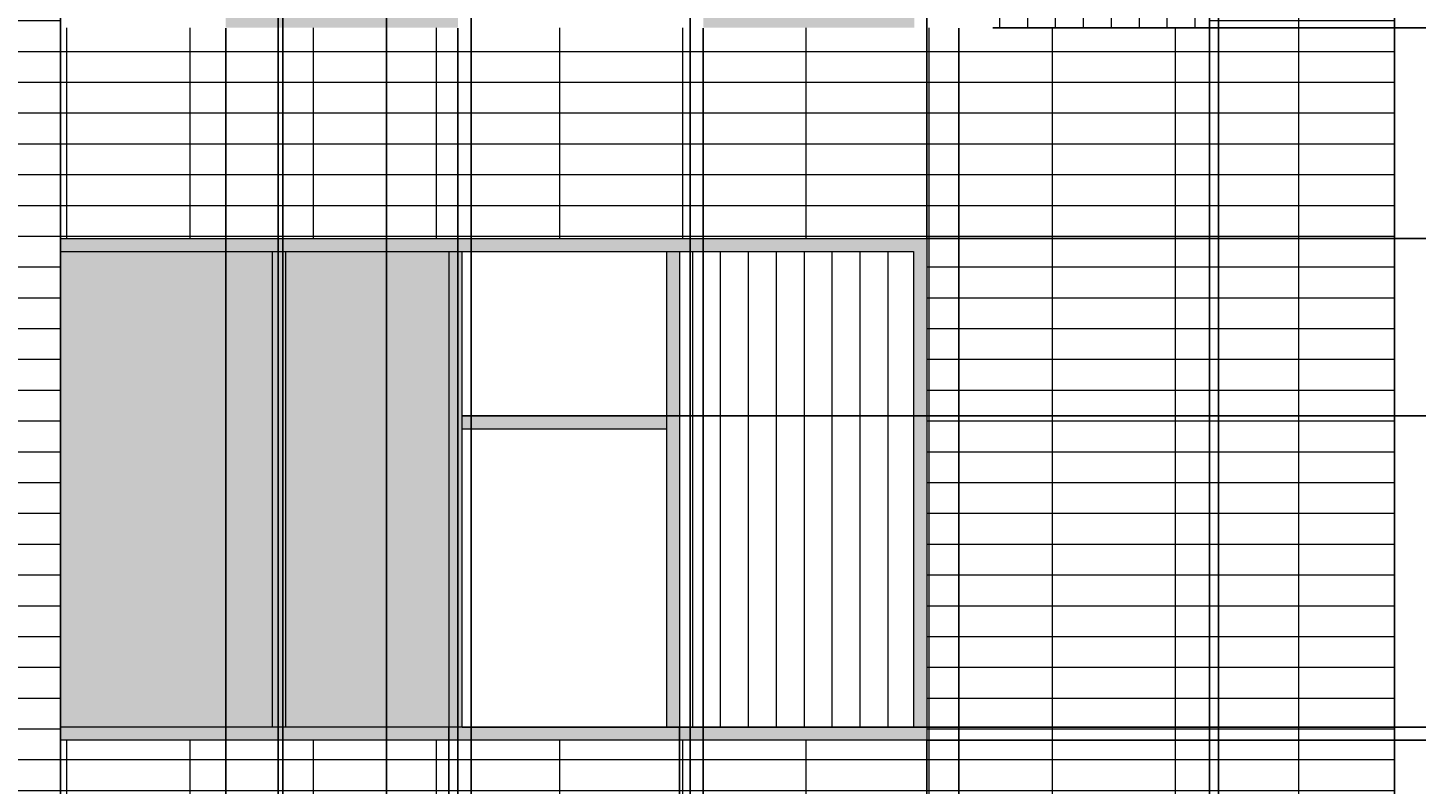
# Model space of a CAD drawing. Units: inches. Extents: x 241 to 943, y 109 to 1396.
# Tile 15 of 34: x 613 to 824, y 620 to 735. Entities that reach past the tile are written whole.
import ezdxf

# ---------------------------------------------------------------- set-up
doc = ezdxf.new("R2010")
doc.units = ezdxf.units.IN
doc.header["$MEASUREMENT"] = 0
for name, color, linetype, lineweight in [('A-ANNO-DIMS', 2, 'Continuous', 18), ('A-ELEV', 7, 'Continuous', 25), ('A-ELEV-SHAD', 9, 'Continuous', 13), ('A-GLAZ', 4, 'Continuous', 18), ('A-GLAZ-PATT', 18, 'Continuous', 13), ('A-WALL-PATT', 8, 'Continuous', 13)]:
    doc.layers.add(name, color=color, linetype=linetype, lineweight=lineweight)
doc.styles.get("Standard").update_dxf_attribs({"font": 'arial.ttf'})
doc.dimstyles.get("Standard").update_dxf_attribs({"dimtxt": 1.4375, "dimasz": 0.18, "dimexe": 0.18, "dimexo": 0.0625, "dimgap": 0.09, "dimtad": 0, "dimtih": 1, "dimtoh": 1, "dimdec": 4, "dimzin": 0, "dimdsep": 46, "dimlunit": 4, "dimtxsty": 'Standard', "dimcen": 0.09, "dimadec": 0, "dimazin": 0, "dimtfac": 1, "dimtdec": 4, "dimtofl": 0, "dimtmove": 0, "dimatfit": 3, "dimfxl": 1, "dimtolj": 1, "dimtzin": 0, "dimarcsym": 0})

# ---------------------------------------------------------------- blocks, each defined once
blk = doc.blocks.new('*D6')
at = {"layer": 'A-ANNO-DIMS', "color": 0, "lineweight": -2, "transparency": 16777216}
for p, q in [((820.84, 232.89), (820.84, 1395.05)), ((881.67, 232.89), (881.67, 1395.05)), ((821.02, 1394.87), (848.73, 1394.87)), ((881.49, 1394.87), (853.77, 1394.87))]:
    blk.add_line(p, q, dxfattribs=at)
at = {"layer": 'A-ANNO-DIMS', "color": 0, "transparency": 16777216}
for points in [[(821.02, 1394.9), (821.02, 1394.84), (820.84, 1394.87)], [(881.49, 1394.9), (881.49, 1394.84), (881.67, 1394.87)]]:
    blk.add_solid(points, dxfattribs=at)
at = {"layer": 'Defpoints', "color": 0, "transparency": 16777216}
for p in [(881.67, 1394.87), (820.84, 232.83), (881.67, 232.83)]:
    blk.add_point(p, dxfattribs=at)
at = {"layer": 'A-ANNO-DIMS', "color": 0, "transparency": 16777216, "insert": (851.25, 1394.87), "char_height": 1.438, "attachment_point": 5}
blk.add_mtext('\\A1;60.83', dxfattribs=at)
blk = doc.blocks.new('*D12')
at = {"layer": 'A-ANNO-DIMS', "color": 0, "lineweight": -2, "transparency": 16777216}
for p, q in [((530.23, 384.24), (530.23, 1395.05)), ((650.91, 384.24), (650.91, 1395.05)), ((530.41, 1394.87), (587.56, 1394.87)), ((650.73, 1394.87), (593.58, 1394.87))]:
    blk.add_line(p, q, dxfattribs=at)
at = {"layer": 'A-ANNO-DIMS', "color": 0, "transparency": 16777216}
for points in [[(530.41, 1394.9), (530.41, 1394.84), (530.23, 1394.87)], [(650.73, 1394.9), (650.73, 1394.84), (650.91, 1394.87)]]:
    blk.add_solid(points, dxfattribs=at)
at = {"layer": 'Defpoints', "color": 0, "transparency": 16777216}
for p in [(650.91, 1394.87), (530.23, 384.18), (650.91, 384.18)]:
    blk.add_point(p, dxfattribs=at)
at = {"layer": 'A-ANNO-DIMS', "color": 0, "transparency": 16777216, "insert": (590.57, 1394.87), "char_height": 1.438, "attachment_point": 5}
blk.add_mtext('\\A1;120.68', dxfattribs=at)
blk = doc.blocks.new('*D13')
at = {"layer": 'A-ANNO-DIMS', "color": 0, "lineweight": -2, "transparency": 16777216}
for p, q in [((650.91, 384.24), (650.91, 1395.05)), ((667.39, 290.06), (667.39, 1395.05)), ((651.09, 1394.87), (656.14, 1394.87)), ((667.21, 1394.87), (662.16, 1394.87))]:
    blk.add_line(p, q, dxfattribs=at)
at = {"layer": 'A-ANNO-DIMS', "color": 0, "transparency": 16777216}
for points in [[(651.09, 1394.9), (651.09, 1394.84), (650.91, 1394.87)], [(667.21, 1394.9), (667.21, 1394.84), (667.39, 1394.87)]]:
    blk.add_solid(points, dxfattribs=at)
at = {"layer": 'Defpoints', "color": 0, "transparency": 16777216}
for p in [(667.39, 1394.87), (650.91, 384.18), (667.39, 290)]:
    blk.add_point(p, dxfattribs=at)
at = {"layer": 'A-ANNO-DIMS', "color": 0, "transparency": 16777216, "insert": (659.15, 1394.87), "char_height": 1.438, "attachment_point": 5}
blk.add_mtext('\\A1;16.486', dxfattribs=at)
blk = doc.blocks.new('*D14')
at = {"layer": 'A-ANNO-DIMS', "color": 0, "lineweight": -2, "transparency": 16777216}
for p, q in [((667.39, 290.06), (667.39, 1395.05)), ((794.03, 290.06), (794.03, 1395.05)), ((667.57, 1394.87), (727.7, 1394.87)), ((793.85, 1394.87), (733.72, 1394.87))]:
    blk.add_line(p, q, dxfattribs=at)
at = {"layer": 'A-ANNO-DIMS', "color": 0, "transparency": 16777216}
for points in [[(667.57, 1394.9), (667.57, 1394.84), (667.39, 1394.87)], [(793.85, 1394.9), (793.85, 1394.84), (794.03, 1394.87)]]:
    blk.add_solid(points, dxfattribs=at)
at = {"layer": 'Defpoints', "color": 0, "transparency": 16777216}
for p in [(794.03, 1394.87), (667.39, 290), (794.03, 290)]:
    blk.add_point(p, dxfattribs=at)
at = {"layer": 'A-ANNO-DIMS', "color": 0, "transparency": 16777216, "insert": (730.71, 1394.87), "char_height": 1.438, "attachment_point": 5}
blk.add_mtext('\\A1;126.63', dxfattribs=at)
blk = doc.blocks.new('*D15')
at = {"layer": 'A-ANNO-DIMS', "color": 0, "lineweight": -2, "transparency": 16777216}
for p, q in [((794.03, 290.06), (794.03, 1395.05)), ((820.84, 232.89), (820.84, 1395.05)), ((794.21, 1394.87), (805.04, 1394.87)), ((820.66, 1394.87), (809.82, 1394.87))]:
    blk.add_line(p, q, dxfattribs=at)
at = {"layer": 'A-ANNO-DIMS', "color": 0, "transparency": 16777216}
for points in [[(794.21, 1394.9), (794.21, 1394.84), (794.03, 1394.87)], [(820.66, 1394.9), (820.66, 1394.84), (820.84, 1394.87)]]:
    blk.add_solid(points, dxfattribs=at)
at = {"layer": 'Defpoints', "color": 0, "transparency": 16777216}
for p in [(820.84, 1394.87), (794.03, 290), (820.84, 232.83)]:
    blk.add_point(p, dxfattribs=at)
at = {"layer": 'A-ANNO-DIMS', "color": 0, "transparency": 16777216, "insert": (807.43, 1394.87), "char_height": 1.438, "attachment_point": 5}
blk.add_mtext('\\A1;26.81', dxfattribs=at)
blk = doc.blocks.new('*D46')
at = {"layer": 'A-ANNO-DIMS', "color": 0, "lineweight": -2, "transparency": 16777216}
for p, q in [((749.7, 702.79), (940.6, 702.79)), ((940.42, 702.61), (940.42, 665.42)), ((940.42, 626.58), (940.42, 663.77)), ((749.7, 626.4), (940.6, 626.4))]:
    blk.add_line(p, q, dxfattribs=at)
at = {"layer": 'A-ANNO-DIMS', "color": 0, "transparency": 16777216}
for points in [[(940.39, 702.61), (940.45, 702.61), (940.42, 702.79)], [(940.39, 626.58), (940.45, 626.58), (940.42, 626.4)]]:
    blk.add_solid(points, dxfattribs=at)
at = {"layer": 'Defpoints', "color": 0, "transparency": 16777216}
for p in [(749.63, 702.79), (940.42, 702.79), (749.63, 626.4)]:
    blk.add_point(p, dxfattribs=at)
at = {"layer": 'A-ANNO-DIMS', "color": 0, "transparency": 16777216, "insert": (940.42, 664.6), "char_height": 1.438, "attachment_point": 5}
blk.add_mtext('\\A1;76.39', dxfattribs=at)
blk = doc.blocks.new('*D47')
at = {"layer": 'A-ANNO-DIMS', "color": 0, "lineweight": -2, "transparency": 16777216}
for p, q in [((792.75, 841.54), (940.6, 841.54)), ((940.42, 841.36), (940.42, 789.02)), ((940.42, 735.03), (940.42, 787.37)), ((792.75, 734.85), (940.6, 734.85))]:
    blk.add_line(p, q, dxfattribs=at)
at = {"layer": 'A-ANNO-DIMS', "color": 0, "transparency": 16777216}
for points in [[(940.39, 841.36), (940.45, 841.36), (940.42, 841.54)], [(940.39, 735.03), (940.45, 735.03), (940.42, 734.85)]]:
    blk.add_solid(points, dxfattribs=at)
at = {"layer": 'Defpoints', "color": 0, "transparency": 16777216}
for p in [(792.69, 841.54), (940.42, 841.54), (792.69, 734.85)]:
    blk.add_point(p, dxfattribs=at)
at = {"layer": 'A-ANNO-DIMS', "color": 0, "transparency": 16777216, "insert": (940.42, 788.2), "char_height": 1.438, "attachment_point": 5}
blk.add_mtext('\\A1;106.68', dxfattribs=at)
blk = doc.blocks.new('*D63')
at = {"layer": 'A-ANNO-DIMS', "color": 0, "lineweight": -2, "transparency": 16777216}
for p, q in [((651.6, 568.89), (651.6, 1395.05)), ((792.69, 568.89), (792.69, 1395.05)), ((651.78, 1394.87), (719.84, 1394.87)), ((792.51, 1394.87), (724.45, 1394.87))]:
    blk.add_line(p, q, dxfattribs=at)
at = {"layer": 'A-ANNO-DIMS', "color": 0, "transparency": 16777216}
for points in [[(651.78, 1394.9), (651.78, 1394.84), (651.6, 1394.87)], [(792.51, 1394.9), (792.51, 1394.84), (792.69, 1394.87)]]:
    blk.add_solid(points, dxfattribs=at)
at = {"layer": 'Defpoints', "color": 0, "transparency": 16777216}
for p in [(792.69, 1394.87), (651.6, 568.83), (792.69, 568.83)]:
    blk.add_point(p, dxfattribs=at)
at = {"layer": 'A-ANNO-DIMS', "color": 0, "transparency": 16777216, "insert": (722.14, 1394.87), "char_height": 1.438, "attachment_point": 5}
blk.add_mtext('\\A1;141.1', dxfattribs=at)
blk = doc.blocks.new('*D64')
at = {"layer": 'A-ANNO-DIMS', "color": 0, "lineweight": -2, "transparency": 16777216}
for p, q in [((792.69, 568.89), (792.69, 1395.05)), ((820.84, 568.89), (820.84, 1395.05)), ((792.87, 1394.87), (803.68, 1394.87)), ((820.66, 1394.87), (809.85, 1394.87))]:
    blk.add_line(p, q, dxfattribs=at)
at = {"layer": 'A-ANNO-DIMS', "color": 0, "transparency": 16777216}
for points in [[(792.87, 1394.9), (792.87, 1394.84), (792.69, 1394.87)], [(820.66, 1394.9), (820.66, 1394.84), (820.84, 1394.87)]]:
    blk.add_solid(points, dxfattribs=at)
at = {"layer": 'Defpoints', "color": 0, "transparency": 16777216}
for p in [(820.84, 1394.87), (792.69, 568.83), (820.84, 568.83)]:
    blk.add_point(p, dxfattribs=at)
at = {"layer": 'A-ANNO-DIMS', "color": 0, "transparency": 16777216, "insert": (806.76, 1394.87), "char_height": 1.438, "attachment_point": 5}
blk.add_mtext('\\A1;28.146', dxfattribs=at)
blk = doc.blocks.new('*D66')
at = {"layer": 'A-ANNO-DIMS', "color": 0, "lineweight": -2, "transparency": 16777216}
for p, q in [((617.76, 702.85), (617.76, 1395.05)), ((749.63, 702.85), (749.63, 1395.05)), ((617.94, 1394.87), (680.69, 1394.87)), ((749.45, 1394.87), (686.7, 1394.87))]:
    blk.add_line(p, q, dxfattribs=at)
at = {"layer": 'A-ANNO-DIMS', "color": 0, "transparency": 16777216}
for points in [[(617.94, 1394.9), (617.94, 1394.84), (617.76, 1394.87)], [(749.45, 1394.9), (749.45, 1394.84), (749.63, 1394.87)]]:
    blk.add_solid(points, dxfattribs=at)
at = {"layer": 'Defpoints', "color": 0, "transparency": 16777216}
for p in [(749.63, 1394.87), (617.76, 702.79), (749.63, 702.79)]:
    blk.add_point(p, dxfattribs=at)
at = {"layer": 'A-ANNO-DIMS', "color": 0, "transparency": 16777216, "insert": (683.7, 1394.87), "char_height": 1.438, "attachment_point": 5}
blk.add_mtext('\\A1;131.87', dxfattribs=at)
blk = doc.blocks.new('*D82')
at = {"layer": 'A-ANNO-DIMS', "color": 0, "lineweight": -2, "transparency": 16777216}
for p, q in [((565.2, 568.89), (565.2, 1395.05)), ((651.6, 568.89), (651.6, 1395.05)), ((565.38, 1394.87), (605.89, 1394.87)), ((651.42, 1394.87), (610.91, 1394.87))]:
    blk.add_line(p, q, dxfattribs=at)
at = {"layer": 'A-ANNO-DIMS', "color": 0, "transparency": 16777216}
for points in [[(565.38, 1394.9), (565.38, 1394.84), (565.2, 1394.87)], [(651.42, 1394.9), (651.42, 1394.84), (651.6, 1394.87)]]:
    blk.add_solid(points, dxfattribs=at)
at = {"layer": 'Defpoints', "color": 0, "transparency": 16777216}
for p in [(651.6, 1394.87), (565.2, 568.83), (651.6, 568.83)]:
    blk.add_point(p, dxfattribs=at)
at = {"layer": 'A-ANNO-DIMS', "color": 0, "transparency": 16777216, "insert": (608.4, 1394.87), "char_height": 1.438, "attachment_point": 5}
blk.add_mtext('\\A1;86.40', dxfattribs=at)
blk = doc.blocks.new('*D83')
at = {"layer": 'A-ANNO-DIMS', "color": 0, "lineweight": -2, "transparency": 16777216}
for p, q in [((592.95, 700.85), (592.95, 1395.05)), ((617.76, 702.85), (617.76, 1395.05)), ((593.13, 1394.87), (602.27, 1394.87)), ((617.58, 1394.87), (608.45, 1394.87))]:
    blk.add_line(p, q, dxfattribs=at)
at = {"layer": 'A-ANNO-DIMS', "color": 0, "transparency": 16777216}
for points in [[(593.13, 1394.9), (593.13, 1394.84), (592.95, 1394.87)], [(617.58, 1394.9), (617.58, 1394.84), (617.76, 1394.87)]]:
    blk.add_solid(points, dxfattribs=at)
at = {"layer": 'Defpoints', "color": 0, "transparency": 16777216}
for p in [(617.76, 1394.87), (617.76, 702.79), (592.95, 700.79)]:
    blk.add_point(p, dxfattribs=at)
at = {"layer": 'A-ANNO-DIMS', "color": 0, "transparency": 16777216, "insert": (605.36, 1394.87), "char_height": 1.438, "attachment_point": 5}
blk.add_mtext('\\A1;24.805', dxfattribs=at)
blk = doc.blocks.new('*D84')
at = {"layer": 'A-ANNO-DIMS', "color": 0, "lineweight": -2, "transparency": 16777216}
for p, q in [((749.63, 702.85), (749.63, 1395.05)), ((820.84, 736.89), (820.84, 1395.05)), ((749.81, 1394.87), (782.73, 1394.87)), ((820.66, 1394.87), (787.74, 1394.87))]:
    blk.add_line(p, q, dxfattribs=at)
at = {"layer": 'A-ANNO-DIMS', "color": 0, "transparency": 16777216}
for points in [[(749.81, 1394.9), (749.81, 1394.84), (749.63, 1394.87)], [(820.66, 1394.9), (820.66, 1394.84), (820.84, 1394.87)]]:
    blk.add_solid(points, dxfattribs=at)
at = {"layer": 'Defpoints', "color": 0, "transparency": 16777216}
for p in [(820.84, 1394.87), (820.84, 736.83), (749.63, 702.79)]:
    blk.add_point(p, dxfattribs=at)
at = {"layer": 'A-ANNO-DIMS', "color": 0, "transparency": 16777216, "insert": (785.24, 1394.87), "char_height": 1.438, "attachment_point": 5}
blk.add_mtext('\\A1;71.20', dxfattribs=at)
blk = doc.blocks.new('*D85')
at = {"layer": 'A-ANNO-DIMS', "color": 0, "lineweight": -2, "transparency": 16777216}
for p, q in [((749.7, 626.4), (940.6, 626.4)), ((940.42, 626.22), (940.42, 598.44)), ((940.42, 569.01), (940.42, 596.79)), ((792.75, 568.83), (940.6, 568.83))]:
    blk.add_line(p, q, dxfattribs=at)
at = {"layer": 'A-ANNO-DIMS', "color": 0, "transparency": 16777216}
for points in [[(940.39, 626.22), (940.45, 626.22), (940.42, 626.4)], [(940.39, 569.01), (940.45, 569.01), (940.42, 568.83)]]:
    blk.add_solid(points, dxfattribs=at)
at = {"layer": 'Defpoints', "color": 0, "transparency": 16777216}
for p in [(749.63, 626.4), (940.42, 626.4), (792.69, 568.83)]:
    blk.add_point(p, dxfattribs=at)
at = {"layer": 'A-ANNO-DIMS', "color": 0, "transparency": 16777216, "insert": (940.42, 597.62), "char_height": 1.438, "attachment_point": 5}
blk.add_mtext('\\A1;57.57', dxfattribs=at)
blk = doc.blocks.new('*D86')
at = {"layer": 'A-ANNO-DIMS', "color": 0, "lineweight": -2, "transparency": 16777216}
for p, q in [((792.75, 734.85), (940.6, 734.85)), ((940.42, 734.67), (940.42, 719.65)), ((940.42, 702.97), (940.42, 718)), ((749.7, 702.79), (940.6, 702.79))]:
    blk.add_line(p, q, dxfattribs=at)
at = {"layer": 'A-ANNO-DIMS', "color": 0, "transparency": 16777216}
for points in [[(940.39, 734.67), (940.45, 734.67), (940.42, 734.85)], [(940.39, 702.97), (940.45, 702.97), (940.42, 702.79)]]:
    blk.add_solid(points, dxfattribs=at)
at = {"layer": 'Defpoints', "color": 0, "transparency": 16777216}
for p in [(792.69, 734.85), (940.42, 734.85), (749.63, 702.79)]:
    blk.add_point(p, dxfattribs=at)
at = {"layer": 'A-ANNO-DIMS', "color": 0, "transparency": 16777216, "insert": (940.42, 718.82), "char_height": 1.438, "attachment_point": 5}
blk.add_mtext('\\A1;32.06', dxfattribs=at)
blk = doc.blocks.new('*D99')
at = {"layer": 'A-ANNO-DIMS', "color": 0, "lineweight": -2, "transparency": 16777216}
for p, q in [((417.09, 181.71), (417.09, 1395.05)), ((667.39, 214.58), (667.39, 1395.05)), ((417.27, 1394.87), (539.16, 1394.87)), ((667.21, 1394.87), (545.33, 1394.87))]:
    blk.add_line(p, q, dxfattribs=at)
at = {"layer": 'A-ANNO-DIMS', "color": 0, "transparency": 16777216}
for points in [[(417.27, 1394.9), (417.27, 1394.84), (417.09, 1394.87)], [(667.21, 1394.9), (667.21, 1394.84), (667.39, 1394.87)]]:
    blk.add_solid(points, dxfattribs=at)
at = {"layer": 'Defpoints', "color": 0, "transparency": 16777216}
for p in [(667.39, 1394.87), (667.39, 214.52), (417.09, 181.65)]:
    blk.add_point(p, dxfattribs=at)
at = {"layer": 'A-ANNO-DIMS', "color": 0, "transparency": 16777216, "insert": (542.24, 1394.87), "char_height": 1.438, "attachment_point": 5}
blk.add_mtext('\\A1;250.30', dxfattribs=at)
blk = doc.blocks.new('*D119')
at = {"layer": 'A-ANNO-DIMS', "color": 0, "lineweight": -2, "transparency": 16777216}
for p, q in [((617.76, 734.79), (617.76, 109.81)), ((642.92, 734.79), (642.92, 109.81)), ((617.94, 109.99), (627.81, 109.99)), ((642.74, 109.99), (632.87, 109.99))]:
    blk.add_line(p, q, dxfattribs=at)
at = {"layer": 'A-ANNO-DIMS', "color": 0, "transparency": 16777216}
for points in [[(617.94, 110.02), (617.94, 109.96), (617.76, 109.99)], [(642.74, 110.02), (642.74, 109.96), (642.92, 109.99)]]:
    blk.add_solid(points, dxfattribs=at)
at = {"layer": 'Defpoints', "color": 0, "transparency": 16777216}
for p in [(617.76, 734.85), (642.92, 734.85), (642.92, 109.99)]:
    blk.add_point(p, dxfattribs=at)
at = {"layer": 'A-ANNO-DIMS', "color": 0, "transparency": 16777216, "insert": (630.34, 109.99), "char_height": 1.438, "attachment_point": 5}
blk.add_mtext('\\A1;25.16', dxfattribs=at)
blk = doc.blocks.new('*D120')
at = {"layer": 'A-ANNO-DIMS', "color": 0, "lineweight": -2, "transparency": 16777216}
for p, q in [((642.92, 734.79), (642.92, 109.81)), ((678.27, 734.79), (678.27, 109.81)), ((643.1, 109.99), (658.07, 109.99)), ((678.09, 109.99), (663.11, 109.99))]:
    blk.add_line(p, q, dxfattribs=at)
at = {"layer": 'A-ANNO-DIMS', "color": 0, "transparency": 16777216}
for points in [[(643.1, 110.02), (643.1, 109.96), (642.92, 109.99)], [(678.09, 110.02), (678.09, 109.96), (678.27, 109.99)]]:
    blk.add_solid(points, dxfattribs=at)
at = {"layer": 'Defpoints', "color": 0, "transparency": 16777216}
for p in [(642.92, 734.85), (678.27, 734.85), (678.27, 109.99)]:
    blk.add_point(p, dxfattribs=at)
at = {"layer": 'A-ANNO-DIMS', "color": 0, "transparency": 16777216, "insert": (660.59, 109.99), "char_height": 1.438, "attachment_point": 5}
blk.add_mtext('\\A1;35.35', dxfattribs=at)
blk = doc.blocks.new('*D121')
at = {"layer": 'A-ANNO-DIMS', "color": 0, "lineweight": -2, "transparency": 16777216}
for p, q in [((680.27, 736.86), (680.27, 109.81)), ((713.62, 736.86), (713.62, 109.81)), ((680.45, 109.99), (693.87, 109.99)), ((713.44, 109.99), (700.02, 109.99))]:
    blk.add_line(p, q, dxfattribs=at)
at = {"layer": 'A-ANNO-DIMS', "color": 0, "transparency": 16777216}
for points in [[(680.45, 110.02), (680.45, 109.96), (680.27, 109.99)], [(713.44, 110.02), (713.44, 109.96), (713.62, 109.99)]]:
    blk.add_solid(points, dxfattribs=at)
at = {"layer": 'Defpoints', "color": 0, "transparency": 16777216}
for p in [(680.27, 736.92), (713.62, 736.92), (713.62, 109.99)]:
    blk.add_point(p, dxfattribs=at)
at = {"layer": 'A-ANNO-DIMS', "color": 0, "transparency": 16777216, "insert": (696.95, 109.99), "char_height": 1.438, "attachment_point": 5}
blk.add_mtext('\\A1;33.356', dxfattribs=at)
blk = doc.blocks.new('*D122')
at = {"layer": 'A-ANNO-DIMS', "color": 0, "lineweight": -2, "transparency": 16777216}
for p, q in [((715.62, 734.79), (715.62, 109.81)), ((754.54, 734.79), (754.54, 109.81)), ((715.8, 109.99), (732.7, 109.99)), ((754.36, 109.99), (737.46, 109.99))]:
    blk.add_line(p, q, dxfattribs=at)
at = {"layer": 'A-ANNO-DIMS', "color": 0, "transparency": 16777216}
for points in [[(715.8, 110.02), (715.8, 109.96), (715.62, 109.99)], [(754.36, 110.02), (754.36, 109.96), (754.54, 109.99)]]:
    blk.add_solid(points, dxfattribs=at)
at = {"layer": 'Defpoints', "color": 0, "transparency": 16777216}
for p in [(715.62, 734.85), (754.54, 734.85), (754.54, 109.99)]:
    blk.add_point(p, dxfattribs=at)
at = {"layer": 'A-ANNO-DIMS', "color": 0, "transparency": 16777216, "insert": (735.08, 109.99), "char_height": 1.438, "attachment_point": 5}
blk.add_mtext('\\A1;38.91', dxfattribs=at)
blk = doc.blocks.new('*D123')
at = {"layer": 'A-ANNO-DIMS', "color": 0, "lineweight": -2, "transparency": 16777216}
for p, q in [((754.54, 734.79), (754.54, 109.81)), ((792.69, 734.79), (792.69, 109.81)), ((754.72, 109.99), (771.09, 109.99)), ((792.51, 109.99), (776.13, 109.99))]:
    blk.add_line(p, q, dxfattribs=at)
at = {"layer": 'A-ANNO-DIMS', "color": 0, "transparency": 16777216}
for points in [[(754.72, 110.02), (754.72, 109.96), (754.54, 109.99)], [(792.51, 110.02), (792.51, 109.96), (792.69, 109.99)]]:
    blk.add_solid(points, dxfattribs=at)
at = {"layer": 'Defpoints', "color": 0, "transparency": 16777216}
for p in [(754.54, 734.85), (792.69, 734.85), (792.69, 109.99)]:
    blk.add_point(p, dxfattribs=at)
at = {"layer": 'A-ANNO-DIMS', "color": 0, "transparency": 16777216, "insert": (773.61, 109.99), "char_height": 1.438, "attachment_point": 5}
blk.add_mtext('\\A1;38.15', dxfattribs=at)
blk = doc.blocks.new('*D125')
at = {"layer": 'A-ANNO-DIMS', "color": 0, "lineweight": -2, "transparency": 16777216}
for p, q in [((754.6, 799.98), (940.6, 799.98)), ((940.42, 799.8), (940.42, 768.24)), ((940.42, 735.03), (940.42, 766.59)), ((759.69, 734.85), (940.6, 734.85))]:
    blk.add_line(p, q, dxfattribs=at)
at = {"layer": 'A-ANNO-DIMS', "color": 0, "transparency": 16777216}
for points in [[(940.39, 799.8), (940.45, 799.8), (940.42, 799.98)], [(940.39, 735.03), (940.45, 735.03), (940.42, 734.85)]]:
    blk.add_solid(points, dxfattribs=at)
at = {"layer": 'Defpoints', "color": 0, "transparency": 16777216}
for p in [(754.54, 799.98), (940.42, 799.98), (759.62, 734.85)]:
    blk.add_point(p, dxfattribs=at)
at = {"layer": 'A-ANNO-DIMS', "color": 0, "transparency": 16777216, "insert": (940.42, 767.42), "char_height": 1.438, "attachment_point": 5}
blk.add_mtext('\\A1;65.13', dxfattribs=at)
blk = doc.blocks.new('*D132')
at = {"layer": 'A-ANNO-DIMS', "color": 0, "lineweight": -2, "transparency": 16777216}
for p, q in [((676.87, 628.34), (676.87, 109.81)), ((617.76, 626.34), (617.76, 109.81)), ((617.94, 109.99), (644.94, 109.99)), ((676.69, 109.99), (649.69, 109.99))]:
    blk.add_line(p, q, dxfattribs=at)
at = {"layer": 'A-ANNO-DIMS', "color": 0, "transparency": 16777216}
for points in [[(617.94, 110.02), (617.94, 109.96), (617.76, 109.99)], [(676.69, 110.02), (676.69, 109.96), (676.87, 109.99)]]:
    blk.add_solid(points, dxfattribs=at)
at = {"layer": 'Defpoints', "color": 0, "transparency": 16777216}
for p in [(676.87, 628.4), (617.76, 626.4), (676.87, 109.99)]:
    blk.add_point(p, dxfattribs=at)
at = {"layer": 'A-ANNO-DIMS', "color": 0, "transparency": 16777216, "insert": (647.31, 109.99), "char_height": 1.438, "attachment_point": 5}
blk.add_mtext('\\A1;59.11', dxfattribs=at)
blk = doc.blocks.new('*D133')
at = {"layer": 'A-ANNO-DIMS', "color": 0, "lineweight": -2, "transparency": 16777216}
for p, q in [((676.87, 628.34), (676.87, 109.81)), ((712.02, 628.34), (712.02, 109.81)), ((677.05, 109.99), (691.92, 109.99)), ((711.84, 109.99), (696.96, 109.99))]:
    blk.add_line(p, q, dxfattribs=at)
at = {"layer": 'A-ANNO-DIMS', "color": 0, "transparency": 16777216}
for points in [[(677.05, 110.02), (677.05, 109.96), (676.87, 109.99)], [(711.84, 110.02), (711.84, 109.96), (712.02, 109.99)]]:
    blk.add_solid(points, dxfattribs=at)
at = {"layer": 'Defpoints', "color": 0, "transparency": 16777216}
for p in [(676.87, 628.4), (712.02, 628.4), (712.02, 109.99)]:
    blk.add_point(p, dxfattribs=at)
at = {"layer": 'A-ANNO-DIMS', "color": 0, "transparency": 16777216, "insert": (694.44, 109.99), "char_height": 1.438, "attachment_point": 5}
blk.add_mtext('\\A1;35.15', dxfattribs=at)
blk = doc.blocks.new('*D134')
at = {"layer": 'A-ANNO-DIMS', "color": 0, "lineweight": -2, "transparency": 16777216}
for p, q in [((712.02, 628.34), (712.02, 109.81)), ((749.63, 626.34), (749.63, 109.81)), ((712.2, 109.99), (727.75, 109.99)), ((749.45, 109.99), (733.9, 109.99))]:
    blk.add_line(p, q, dxfattribs=at)
at = {"layer": 'A-ANNO-DIMS', "color": 0, "transparency": 16777216}
for points in [[(712.2, 110.02), (712.2, 109.96), (712.02, 109.99)], [(749.45, 110.02), (749.45, 109.96), (749.63, 109.99)]]:
    blk.add_solid(points, dxfattribs=at)
at = {"layer": 'Defpoints', "color": 0, "transparency": 16777216}
for p in [(712.02, 628.4), (749.63, 626.4), (749.63, 109.99)]:
    blk.add_point(p, dxfattribs=at)
at = {"layer": 'A-ANNO-DIMS', "color": 0, "transparency": 16777216, "insert": (730.82, 109.99), "char_height": 1.438, "attachment_point": 5}
blk.add_mtext('\\A1;37.616', dxfattribs=at)
blk = doc.blocks.new('*D135')
at = {"layer": 'A-ANNO-DIMS', "color": 0, "lineweight": -2, "transparency": 16777216}
for p, q in [((678.93, 675.79), (940.6, 675.79)), ((940.42, 675.61), (940.42, 652.92)), ((940.42, 628.58), (940.42, 651.27)), ((678.93, 628.4), (940.6, 628.4))]:
    blk.add_line(p, q, dxfattribs=at)
at = {"layer": 'A-ANNO-DIMS', "color": 0, "transparency": 16777216}
for points in [[(940.39, 675.61), (940.45, 675.61), (940.42, 675.79)], [(940.39, 628.58), (940.45, 628.58), (940.42, 628.4)]]:
    blk.add_solid(points, dxfattribs=at)
at = {"layer": 'Defpoints', "color": 0, "transparency": 16777216}
for p in [(678.87, 675.79), (940.42, 675.79), (678.87, 628.4)]:
    blk.add_point(p, dxfattribs=at)
at = {"layer": 'A-ANNO-DIMS', "color": 0, "transparency": 16777216, "insert": (940.42, 652.09), "char_height": 1.438, "attachment_point": 5}
blk.add_mtext('\\A1;47.38', dxfattribs=at)

msp = doc.modelspace()

# ---------------------------------------------------------------- hatches: boundary and pattern name
at = {"layer": 'A-ELEV-SHAD'}
h = msp.add_hatch(color=256, dxfattribs=at)
h.dxf.hatch_style = 1
h.paths.add_polyline_path([(537.4269, 566.8295), (534.1778, 566.8295), (534.1778, 527.3816), (537.4269, 527.3816)])
h.paths.add_polyline_path([(508.0803, 566.8295), (450.9259, 566.8295), (450.9259, 527.3816), (452.9259, 527.3816), (452.9259, 564.8295), (506.0803, 564.8295), (506.0803, 527.3816), (508.0803, 527.3816)])
h.paths.add_polyline_path([(481.5031, 564.8295), (479.5031, 564.8295), (479.5031, 527.3816), (481.5031, 527.3816)], flags=17)
h.paths.add_polyline_path([(481.5031, 525.3816), (479.5031, 525.3816), (479.5031, 521.3754), (481.5031, 521.3754)], flags=17)
h.paths.add_polyline_path([(508.0803, 525.3816), (506.0803, 525.3816), (506.0803, 521.3754), (452.9259, 521.3754), (452.9259, 525.3816), (450.9259, 525.3816), (450.9259, 519.3754), (508.0803, 519.3754)])
h.paths.add_polyline_path([(537.4269, 525.3816), (534.1778, 525.3816), (534.1778, 508.9074), (537.4269, 508.9074)])
h.paths.add_polyline_path([(749.6328, 702.7912), (617.7594, 702.7912), (617.7594, 700.7912), (747.6328, 700.7912), (747.6328, 628.4013), (617.7594, 628.4013), (617.7594, 626.4013), (749.6328, 626.4013)])
h.paths.add_polyline_path([(652.0129, 700.7912), (650.0129, 700.7912), (650.0129, 628.4013), (652.0129, 628.4013)], flags=17)
h.paths.add_polyline_path([(678.8698, 700.7912), (676.8698, 700.7912), (676.8698, 628.4013), (678.8698, 628.4013)], flags=17)
h.paths.add_polyline_path([(712.0171, 700.7912), (710.0171, 700.7912), (710.0171, 628.4013), (712.0171, 628.4013)], flags=17)
h.paths.add_polyline_path([(710.0171, 675.7856), (678.8698, 675.7856), (678.8698, 673.7856), (710.0171, 673.7856)], flags=17)
h.paths.add_polyline_path([(537.4269, 698.7912), (534.1778, 698.7912), (534.1778, 659.3434), (537.4269, 659.3434)], flags=0)
h.paths.add_polyline_path([(592.9542, 700.7912), (424.1086, 700.7912), (424.1086, 628.4013), (592.9542, 628.4013)])
h.paths.add_polyline_path([(590.8792, 698.7912), (590.8792, 630.4013), (426.1086, 630.4013), (426.1086, 698.7912)], flags=16)
h.paths.add_polyline_path([(563.2023, 698.7912), (563.2023, 659.3434), (563.9297, 659.3434), (563.9297, 651.3371), (508.1906, 651.3371), (508.0803, 651.3371), (450.9259, 651.3371), (428.0291, 651.3371), (428.0291, 698.7912), (451.9767, 698.7912), (508.0803, 698.7912), (537.4269, 698.7912)], flags=0)
h.paths.add_polyline_path([(506.0803, 696.7912), (506.0803, 653.3371), (452.9259, 653.3371), (452.9259, 657.3434), (445.5808, 657.3434, -1), (445.5808, 659.3434), (452.9259, 659.3434), (452.9259, 696.7912)], flags=0)
h.paths.add_polyline_path([(563.9297, 698.7912), (563.2023, 698.7912), (563.2023, 659.3434), (563.9297, 659.3434)], flags=0)
at = {"layer": 'A-GLAZ-PATT'}
h = msp.add_hatch(dxfattribs=at)
h.set_pattern_fill('GOST_GLASS', color=256, scale=0.89)
h.set_pattern_definition([(45, (0, 0), (7.5519, 0), [4.45, -6.23]), (45, (1.888, 0), (7.5519, 0), [1.78, -8.9]), (45, (0, 1.888), (7.5519, 0), [1.78, -8.9])])
h.paths.add_polyline_path([(676.8698, 700.7912), (652.0129, 700.7912), (652.0129, 628.4013), (676.8698, 628.4013)])
h.paths.add_polyline_path([(650.0129, 700.7912), (617.7594, 700.7912), (617.7594, 628.4013), (650.0129, 628.4013)])
h.paths.add_polyline_path([(747.7579, 841.5382), (715.6236, 841.5382), (715.6236, 734.8538), (747.7579, 734.8538)])
h.paths.add_polyline_path([(678.2674, 841.5382), (642.9197, 841.5382), (642.9197, 734.8538), (678.2674, 734.8538)])
h.paths.add_polyline_path([(712.5839, 1009.5382), (677.6886, 1009.5382), (677.6886, 902.8538), (712.5839, 902.8538)])
h.paths.add_polyline_path([(640.1141, 1009.5382), (603.8694, 1009.5382), (603.8694, 902.8538), (640.1141, 902.8538)])
h.paths.add_polyline_path([(682.8748, 1175.7336), (643.4534, 1175.7336), (643.4534, 1110.1686), (682.8748, 1110.1686)])
h.paths.add_polyline_path([(602.3616, 1175.7336), (565.947, 1175.7336), (565.947, 1110.1686), (602.3616, 1110.1686)])
h = msp.add_hatch(dxfattribs=at)
h.set_pattern_fill('ANSI31', color=256, scale=34, angle=45)
h.paths.add_polyline_path([(486.3418, 786.9154), (413.1187, 786.9154), (413.1187, 761.2284), (486.3418, 761.2284)])
h.paths.add_polyline_path([(486.3418, 954.9154), (413.1187, 954.9154), (413.1187, 929.2284), (486.3418, 929.2284)])
h.paths.add_polyline_path([(462.1074, 289.6933), (390.895, 289.6933), (390.895, 277.4626), (390.895, 274.3507), (462.1074, 274.3507), (462.1074, 277.4626)])
h.paths.add_polyline_path([(500.3323, 289.6933), (479.596, 289.6933), (479.596, 274.3507), (500.3323, 274.3507)])
h.paths.add_polyline_path([(450.9259, 566.8295), (426.1086, 566.8295), (426.1086, 498.4395), (446.4348, 498.4395), (446.4348, 519.3754), (450.9259, 519.3754), (450.9259, 525.3816), (445.5808, 525.3816, -1), (445.5808, 527.3816), (450.9259, 527.3816)])
h.paths.add_polyline_path([(563.2023, 508.9074), (534.1778, 508.9074), (508.1906, 508.9074), (508.1906, 498.4395), (563.2023, 498.4395)])
h.paths.add_polyline_path([(747.6328, 700.7912), (712.0171, 700.7912), (712.0171, 628.4013), (747.6328, 628.4013)])
h.paths.add_polyline_path([(446.4348, 643.7483), (426.1086, 643.7483), (426.1086, 630.4013), (446.4348, 630.4013)])
h.paths.add_polyline_path([(564.8076, 841.5382), (553.5166, 841.5382), (508.3064, 841.5382), (508.3064, 782.5808), (564.8076, 782.5808)])
h.paths.add_polyline_path([(564.8076, 780.5808), (508.3064, 780.5808), (508.3064, 773.4916), (564.8076, 773.4916)])
h.paths.add_polyline_path([(792.691, 762.5799), (759.6248, 762.5799), (759.6248, 736.9235), (759.6248, 734.8538), (792.691, 734.8538)])
h.paths.add_polyline_path([(564.8076, 1009.5382), (553.5166, 1009.5382), (508.3064, 1009.5382), (508.3064, 950.5808), (562.3033, 950.5808, -1), (562.3033, 948.5808), (508.3064, 948.5808), (508.3064, 941.4916), (564.8076, 941.4916)])
h.paths.add_polyline_path([(486.3418, 1122.9154), (413.1187, 1122.9154), (413.1187, 1097.2284), (486.3418, 1097.2284)])
at = {"layer": 'A-WALL-PATT'}
h = msp.add_hatch(dxfattribs=at)
h.set_pattern_fill('GRATE', color=256, scale=150)
h.paths.add_polyline_path([(747.7579, 1238.8538), (747.7579, 1275.9142), (747.7579, 1336.1154), (508.3064, 1336.1154), (508.3064, 1275.9142), (508.3064, 1238.8538), (508.3064, 1177.5382), (508.3064, 1109.4916), (508.3064, 1070.8538), (553.5166, 1070.8538), (749.6328, 1070.8538)])
h.paths.add_polyline_path([(533.952, 1108.1686), (533.952, 1177.7336), (533.952, 1303.0286), (724.819, 1303.0286), (724.819, 1108.1686)], flags=16)
h.paths.add_polyline_path([(535.952, 1110.1686), (535.952, 1175.7336), (722.819, 1175.7336), (722.819, 1110.1686)], flags=0)
h.paths.add_polyline_path([(643.4534, 1134.0739), (622.521, 1134.0739), (622.521, 1136.0739), (643.4534, 1136.0739)], flags=0)
h.paths.add_polyline_path([(617.7594, 568.8295), (617.7594, 734.8538), (377.0391, 734.8538), (377.0391, 566.8538), (377.0391, 400.8295), (417.0913, 400.8295), (618.9643, 400.8295)])
h.paths.add_polyline_path([(424.1086, 496.4395), (424.1086, 568.8295), (565.2023, 568.8295), (565.2023, 496.4395)], flags=16)
h.paths.add_polyline_path([(426.1086, 498.4395), (426.1086, 566.8295), (563.2023, 566.8295), (563.2023, 508.9074), (563.2023, 498.4395)], flags=0)
h.paths.add_polyline_path([(508.0803, 508.9074), (508.0803, 519.3754), (450.9259, 519.3754), (450.9259, 525.3816), (445.5808, 525.3816, -1), (445.5808, 527.3816), (450.9259, 527.3816), (450.9259, 566.8295), (508.0803, 566.8295), (537.4269, 566.8295), (537.4269, 508.9074)], flags=0)
h.paths.add_polyline_path([(506.0803, 521.3754), (452.9259, 521.3754), (452.9259, 564.8295), (506.0803, 564.8295)], flags=0)
h.paths.add_polyline_path([(424.1086, 628.4013), (424.1086, 700.7912), (592.9542, 700.7912), (592.9542, 628.4013)], flags=16)
h.paths.add_polyline_path([(426.1086, 630.4013), (426.1086, 698.7912), (590.8792, 698.7912), (590.8792, 630.4013)], flags=0)
h.paths.add_polyline_path([(508.1906, 651.3371), (508.0803, 651.3371), (450.9259, 651.3371), (428.0291, 651.3371), (428.0291, 698.7912), (451.9767, 698.7912), (508.0803, 698.7912), (537.4269, 698.7912), (563.2023, 698.7912), (563.2023, 659.3434), (563.9297, 659.3434), (563.9297, 651.3371)], flags=0)
h.paths.add_polyline_path([(506.0803, 653.3371), (452.9259, 653.3371), (452.9259, 657.3434), (445.5808, 657.3434, -1), (445.5808, 659.3434), (452.9259, 659.3434), (452.9259, 696.7912), (506.0803, 696.7912)], flags=0)
h = msp.add_hatch(dxfattribs=at)
h.set_pattern_fill('GRATE', color=256, scale=150)
h.paths.add_polyline_path([(820.8374, 1070.8538), (749.6328, 1070.8538), (553.5166, 1070.8538), (508.3064, 1070.8538), (508.3064, 1009.5382), (553.5166, 1009.5382), (564.8076, 1009.5382), (603.8694, 1009.5382), (751.5078, 1009.5382), (751.5078, 902.8538), (603.8694, 902.8538), (603.8694, 1009.5382), (564.8076, 1009.5382), (564.8076, 941.4916), (568.1348, 941.4916), (568.1348, 902.8538), (581.3632, 902.8538), (581.3632, 841.5382), (564.8076, 841.5382), (564.8076, 782.5808), (605.9087, 782.5808, -1), (605.9087, 780.5808), (564.8076, 780.5808), (564.8076, 773.4916), (597.514, 773.4916), (607.8162, 773.4916), (607.8162, 734.8538), (617.7594, 734.8538), (617.7594, 841.5382), (792.691, 841.5382), (792.691, 734.8538), (617.7594, 734.8538), (617.7594, 702.7912), (749.6328, 702.7912), (749.6328, 626.4013), (617.7594, 626.4013), (617.7594, 568.8295), (820.8374, 568.8295), (820.8374, 736.8295), (820.8374, 902.8538)])

# ---------------------------------------------------------------- linework, layer by layer
at = {"layer": 'A-ELEV'}
for p, q in [((820.8374, 568.8295), (820.8374, 736.8295)), ((617.7594, 568.8295), (617.7594, 734.8538))]:
    msp.add_line(p, q, dxfattribs=at)
at = {"layer": 'A-GLAZ'}
for p, q in [((650.0129, 700.7912), (650.0129, 628.4013)), ((652.0129, 700.7912), (652.0129, 628.4013)), ((676.8698, 700.7912), (676.8698, 628.4013)), ((678.8698, 700.7912), (678.8698, 628.4013)), ((710.0171, 700.7912), (710.0171, 628.4013)), ((712.0171, 700.7912), (712.0171, 628.4013)), ((678.8698, 675.7856), (710.0171, 675.7856)), ((678.8698, 673.7856), (710.0171, 673.7856))]:
    msp.add_line(p, q, dxfattribs=at)
msp.add_lwpolyline([(617.7594, 702.7912), (749.6328, 702.7912), (749.6328, 626.4013), (617.7594, 626.4013)], dxfattribs=at)
msp.add_lwpolyline([(617.7594, 700.7912), (747.6328, 700.7912), (747.6328, 628.4013), (617.7594, 628.4013)], close=True, dxfattribs=at)

# ---------------------------------------------------------------- dimensions: what is measured, and where the dimension line sits
at = {"layer": 'A-ANNO-DIMS'}
for base, p1, p2, override, picture, middle in [((667.3935, 1394.8654), (417.0913, 181.649), (667.3935, 214.5189), {"dimdec": 2, "dimlfac": 1, "dimrnd": 0, "dimzin": 0, "dimdsep": 46, "dimlunit": 2}, '*D99', (542.2424, 1394.8654)), ((650.907, 1394.8654), (530.2303, 384.1784), (650.907, 384.1784), {"dimdec": 2, "dimlfac": 1, "dimrnd": 0, "dimzin": 0, "dimdsep": 46, "dimlunit": 2}, '*D12', (590.5686, 1394.8654)), ((651.5974, 1394.8654), (565.2023, 568.8295), (651.5974, 568.8295), {"dimdec": 2, "dimlfac": 1, "dimrnd": 0, "dimzin": 0, "dimdsep": 46, "dimlunit": 2}, '*D82', (608.3998, 1394.8654)), ((617.7594, 1394.8654), (592.9542, 700.7912), (617.7594, 702.7912), {"dimdec": 3, "dimlfac": 1, "dimrnd": 0, "dimzin": 0, "dimdsep": 46, "dimlunit": 2}, '*D83', (605.3568, 1394.8654)), ((749.6328, 1394.8654), (617.7594, 702.7912), (749.6328, 702.7912), {"dimdec": 2, "dimlfac": 1, "dimrnd": 0, "dimzin": 0, "dimdsep": 46, "dimlunit": 2}, '*D66', (683.6961, 1394.8654)), ((667.39345, 1394.86544), (650.90697, 384.17836), (667.39345, 289.99842), {"dimdec": 3, "dimlfac": 1, "dimrnd": 0, "dimzin": 0, "dimdsep": 46, "dimlunit": 2}, '*D13', (659.15021, 1394.86544)), ((792.691, 1394.8654), (651.5974, 568.8295), (792.691, 568.8295), {"dimdec": 1, "dimlfac": 1, "dimrnd": 0, "dimzin": 0, "dimdsep": 46, "dimlunit": 2}, '*D63', (722.1442, 1394.8654)), ((794.0275, 1394.8654), (667.3935, 289.9984), (794.0275, 289.9984), {"dimdec": 2, "dimlfac": 1, "dimrnd": 0, "dimzin": 0, "dimdsep": 46, "dimlunit": 2}, '*D14', (730.7105, 1394.8654)), ((820.8374, 1394.8654), (749.6328, 702.7912), (820.8374, 736.8295), {"dimdec": 2, "dimlfac": 1, "dimrnd": 0, "dimzin": 0, "dimdsep": 46, "dimlunit": 2}, '*D84', (785.2351, 1394.8654)), ((820.8374, 1394.8654), (792.691, 568.8295), (820.8374, 568.8295), {"dimdec": 3, "dimlfac": 1, "dimrnd": 0, "dimzin": 0, "dimdsep": 46, "dimlunit": 2}, '*D64', (806.7642, 1394.8654)), ((820.8374, 1394.8654), (794.0275, 289.9984), (820.8374, 232.8295), {"dimdec": 2, "dimlfac": 1, "dimrnd": 0, "dimzin": 0, "dimdsep": 46, "dimlunit": 2}, '*D15', (807.4324, 1394.8654)), ((881.667, 1394.8654), (820.8374, 232.8295), (881.667, 232.8295), {"dimdec": 2, "dimlfac": 1, "dimrnd": 0, "dimzin": 0, "dimdsep": 46, "dimlunit": 2}, '*D6', (851.2522, 1394.8654)), ((713.6236, 109.9907), (680.2674, 736.9235), (713.6236, 736.9235), {"dimdec": 3, "dimlfac": 1, "dimrnd": 0, "dimzin": 0, "dimdsep": 46, "dimlunit": 2}, '*D121', (696.9455, 109.9907)), ((642.9197, 109.9907), (617.7594, 734.8538), (642.9197, 734.8538), {"dimdec": 2, "dimlfac": 1, "dimrnd": 0, "dimzin": 0, "dimdsep": 46, "dimlunit": 2}, '*D119', (630.3395, 109.9907)), ((678.2674, 109.9907), (642.9197, 734.8538), (678.2674, 734.8538), {"dimdec": 2, "dimlfac": 1, "dimrnd": 0, "dimzin": 0, "dimdsep": 46, "dimlunit": 2}, '*D120', (660.5935, 109.9907)), ((754.5373, 109.9907), (715.6236, 734.8538), (754.5373, 734.8538), {"dimdec": 2, "dimlfac": 1, "dimrnd": 0, "dimzin": 0, "dimdsep": 46, "dimlunit": 2}, '*D122', (735.0804, 109.9907)), ((792.691, 109.9907), (754.5373, 734.8538), (792.691, 734.8538), {"dimdec": 2, "dimlfac": 1, "dimrnd": 0, "dimzin": 0, "dimdsep": 46, "dimlunit": 2}, '*D123', (773.6142, 109.9907)), ((676.8698, 109.9907), (617.7594, 626.4013), (676.8698, 628.4013), {"dimdec": 2, "dimlfac": 1, "dimrnd": 0, "dimzin": 0, "dimdsep": 46, "dimlunit": 2}, '*D132', (647.3146, 109.9907)), ((712.0171, 109.9907), (676.8698, 628.4013), (712.0171, 628.4013), {"dimdec": 2, "dimlfac": 1, "dimrnd": 0, "dimzin": 0, "dimdsep": 46, "dimlunit": 2}, '*D133', (694.4435, 109.9907)), ((749.6328, 109.9907), (712.0171, 628.4013), (749.6328, 626.4013), {"dimdec": 3, "dimlfac": 1, "dimrnd": 0, "dimzin": 0, "dimdsep": 46, "dimlunit": 2}, '*D134', (730.825, 109.9907))]:
    dim = msp.add_linear_dim(base=base, p1=p1, p2=p2, dimstyle='Standard', override=override, dxfattribs=at)
    dim.commit()
    dim.dimension.update_dxf_attribs({"geometry": picture, "text_midpoint": middle})
for base, p1, p2, picture, middle in [((940.417, 841.5382), (792.691, 734.8538), (792.691, 841.5382), '*D47', (940.417, 788.196)), ((940.417, 799.9791), (759.6248, 734.8538), (754.5373, 799.9791), '*D125', (940.417, 767.4165)), ((940.417, 734.8538), (749.6328, 702.7912), (792.691, 734.8538), '*D86', (940.417, 718.8225)), ((940.417, 702.7912), (749.6328, 626.4013), (749.6328, 702.7912), '*D46', (940.417, 664.5962)), ((940.417, 675.7856), (678.8698, 628.4013), (678.8698, 675.7856), '*D135', (940.417, 652.0934)), ((940.417, 626.4013), (792.691, 568.8295), (749.6328, 626.4013), '*D85', (940.417, 597.6154))]:
    dim = msp.add_linear_dim(base=base, p1=p1, p2=p2, angle=90, dimstyle='Standard', override={"dimdec": 2, "dimlfac": 1, "dimrnd": 0, "dimzin": 0, "dimdsep": 46, "dimlunit": 2}, dxfattribs=at)
    dim.commit()
    dim.dimension.update_dxf_attribs({"geometry": picture, "text_midpoint": middle})

doc.saveas('drawing.dxf')
